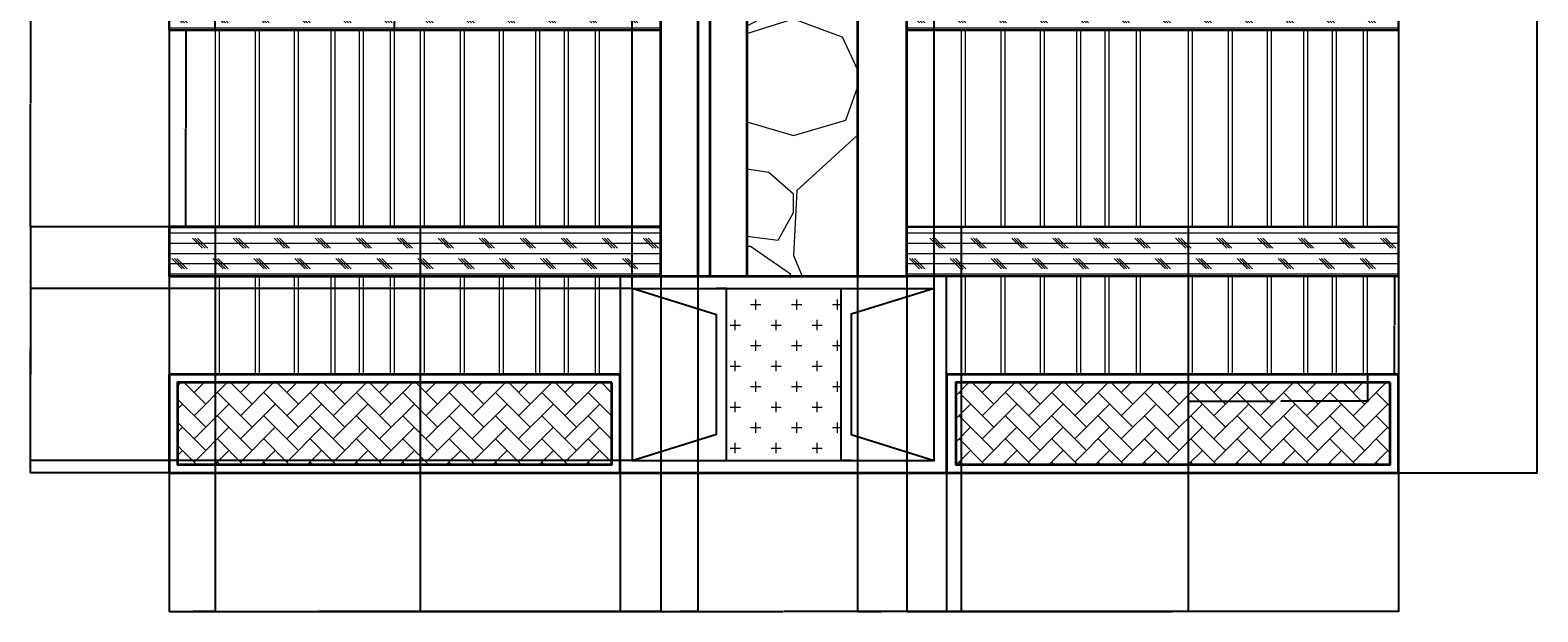
# Model space of a CAD drawing. Units: inches. Extents: x -38 to 698, y -57 to 1364.
# Tile 1 of 5: x -38 to 698, y -57 to 227. Entities that reach past the tile are written whole.
import ezdxf

# ---------------------------------------------------------------- set-up
doc = ezdxf.new("R2010")
doc.units = ezdxf.units.IN
doc.header["$MEASUREMENT"] = 0
for name, color, linetype, lineweight in [('A-ANNO-DIMS', 2, 'Continuous', 18), ('A-DOOR', 3, 'Continuous', 25), ('A-DOOR-PATT', 8, 'Continuous', 13), ('A-ELEV-PATT', 8, 'Continuous', 13), ('A-ELEV-SCRN', 7, 'Continuous', 20), ('A-FLOR', 7, 'Continuous', 30), ('A-WALL', 7, 'Continuous', 35), ('A-WALL-PATT', 8, 'Continuous', 13)]:
    doc.layers.add(name, color=color, linetype=linetype, lineweight=lineweight)
doc.styles.get("Standard").update_dxf_attribs({"font": 'arial.ttf'})
doc.dimstyles.get("Standard").update_dxf_attribs({"dimtxt": 0.18, "dimasz": 0.18, "dimexe": 0.18, "dimexo": 0.0625, "dimgap": 0.09, "dimtad": 0, "dimtih": 1, "dimtoh": 1, "dimdec": 4, "dimzin": 0, "dimdsep": 46, "dimtxsty": 'Standard', "dimcen": 0.09, "dimadec": 0, "dimazin": 0, "dimtfac": 1, "dimtdec": 4, "dimtofl": 0, "dimtmove": 0, "dimatfit": 3, "dimfxl": 1, "dimtolj": 1, "dimtzin": 0, "dimarcsym": 0})

# ---------------------------------------------------------------- blocks, each defined once
blk = doc.blocks.new('PODIUM-SCREEN-48')
for points in [[(0, 0), (2.11, 0), (2.11, 48), (0, 48)], [(19.49, 0), (21.6, 0), (21.6, 48), (19.49, 48)], [(38.57, 0), (40.67, 0), (40.67, 48), (38.57, 48)], [(56.37, 0), (58.48, 0), (58.48, 48), (56.37, 48)], [(70.28, 0), (72.39, 0), (72.39, 48), (70.28, 48)], [(85.45, 0), (87.56, 0), (87.56, 48), (85.45, 48)]]:
    blk.add_lwpolyline(points, close=True)
blk = doc.blocks.new('PODIUM-SCREEN-96')
for points in [[(0, 0), (2.11, 0), (2.11, 96), (0, 96)], [(19.49, 0), (21.6, 0), (21.6, 96), (19.49, 96)], [(38.57, 0), (40.67, 0), (40.67, 96), (38.57, 96)], [(56.37, 0), (58.48, 0), (58.48, 96), (56.37, 96)], [(70.28, 0), (72.39, 0), (72.39, 96), (70.28, 96)], [(85.45, 0), (87.56, 0), (87.56, 96), (85.45, 96)]]:
    blk.add_lwpolyline(points, close=True)
blk = doc.blocks.new('*D18')
at = {"layer": 'A-ANNO-DIMS', "color": 0, "lineweight": -2, "transparency": 16777216}
for p, q in [((527.04, 59.15), (527.04, 45.9)), ((614.61, 59.15), (614.61, 45.9)), ((527.22, 46.08), (569.42, 46.08)), ((614.43, 46.08), (572.23, 46.08))]:
    blk.add_line(p, q, dxfattribs=at)
at = {"layer": 'A-ANNO-DIMS', "color": 0, "transparency": 16777216}
for points in [[(527.22, 46.11), (527.22, 46.05), (527.04, 46.08)], [(614.43, 46.11), (614.43, 46.05), (614.61, 46.08)]]:
    blk.add_solid(points, dxfattribs=at)
at = {"layer": 'Defpoints', "color": 0, "transparency": 16777216}
for p in [(527.04, 59.21), (614.61, 59.21), (614.61, 46.08)]:
    blk.add_point(p, dxfattribs=at)
at = {"layer": 'A-ANNO-DIMS', "color": 0, "transparency": 16777216, "insert": (570.82, 46.08), "char_height": 0.18, "attachment_point": 5}
blk.add_mtext('\\A1;LOW SCREEN 88 TYP.', dxfattribs=at)
blk = doc.blocks.new('*D19')
at = {"layer": 'A-ANNO-DIMS', "color": 0, "lineweight": -2, "transparency": 16777216}
for p, q in [((614.67, 107.21), (627.92, 107.21)), ((627.74, 107.03), (627.74, 83.4)), ((627.74, 59.39), (627.74, 83.03)), ((614.67, 59.21), (627.92, 59.21))]:
    blk.add_line(p, q, dxfattribs=at)
at = {"layer": 'A-ANNO-DIMS', "color": 0, "transparency": 16777216}
for points in [[(627.71, 107.03), (627.77, 107.03), (627.74, 107.21)], [(627.71, 59.39), (627.77, 59.39), (627.74, 59.21)]]:
    blk.add_solid(points, dxfattribs=at)
at = {"layer": 'Defpoints', "color": 0, "transparency": 16777216}
for p in [(614.61, 107.21), (627.74, 107.21), (614.61, 59.21)]:
    blk.add_point(p, dxfattribs=at)
at = {"layer": 'A-ANNO-DIMS', "color": 0, "transparency": 16777216, "insert": (627.74, 83.21), "char_height": 0.18, "attachment_point": 5}
blk.add_mtext('\\A1;48 TYP.', dxfattribs=at)
blk = doc.blocks.new('*D20')
at = {"layer": 'A-ANNO-DIMS', "color": 0, "lineweight": -2, "transparency": 16777216}
for p, q in [((52.08, 227.21), (37.56, 227.21)), ((37.74, 227.03), (37.74, 179.4)), ((37.74, 131.39), (37.74, 179.03)), ((52.08, 131.21), (37.56, 131.21))]:
    blk.add_line(p, q, dxfattribs=at)
at = {"layer": 'A-ANNO-DIMS', "color": 0, "transparency": 16777216}
for points in [[(37.71, 227.03), (37.77, 227.03), (37.74, 227.21)], [(37.71, 131.39), (37.77, 131.39), (37.74, 131.21)]]:
    blk.add_solid(points, dxfattribs=at)
at = {"layer": 'Defpoints', "color": 0, "transparency": 16777216}
for p in [(37.74, 227.21), (52.14, 227.21), (52.14, 131.21)]:
    blk.add_point(p, dxfattribs=at)
at = {"layer": 'A-ANNO-DIMS', "color": 0, "transparency": 16777216, "insert": (37.74, 179.21), "char_height": 0.18, "attachment_point": 5}
blk.add_mtext('\\A1;HIGH SCREEN 96 TYP.', dxfattribs=at)
blk = doc.blocks.new('*D21')
at = {"layer": 'A-ANNO-DIMS', "color": 0, "lineweight": -2, "transparency": 16777216}
for p, q in [((52.14, 227.28), (52.14, 241.79)), ((52.32, 241.61), (95.39, 241.61)), ((139.52, 241.61), (96.45, 241.61)), ((139.7, 227.28), (139.7, 241.79))]:
    blk.add_line(p, q, dxfattribs=at)
at = {"layer": 'A-ANNO-DIMS', "color": 0, "transparency": 16777216}
for points in [[(52.32, 241.64), (52.32, 241.58), (52.14, 241.61)], [(139.52, 241.64), (139.52, 241.58), (139.7, 241.61)]]:
    blk.add_solid(points, dxfattribs=at)
at = {"layer": 'Defpoints', "color": 0, "transparency": 16777216}
for p in [(139.7, 241.61), (52.14, 227.21), (139.7, 227.21)]:
    blk.add_point(p, dxfattribs=at)
at = {"layer": 'A-ANNO-DIMS', "color": 0, "transparency": 16777216, "insert": (95.92, 241.61), "char_height": 0.18, "attachment_point": 5}
blk.add_mtext('\\A1;88 TYP.', dxfattribs=at)
blk = doc.blocks.new('*D22')
at = {"layer": 'A-ANNO-DIMS', "color": 0, "lineweight": -2, "transparency": 16777216}
for p, q in [((29.69, 500.15), (29.69, -56.67)), ((629.69, 500.15), (629.69, -56.67)), ((29.87, -56.49), (329.4, -56.49)), ((629.51, -56.49), (329.97, -56.49))]:
    blk.add_line(p, q, dxfattribs=at)
at = {"layer": 'A-ANNO-DIMS', "color": 0, "transparency": 16777216}
for points in [[(29.87, -56.46), (29.87, -56.52), (29.69, -56.49)], [(629.51, -56.46), (629.51, -56.52), (629.69, -56.49)]]:
    blk.add_solid(points, dxfattribs=at)
at = {"layer": 'Defpoints', "color": 0, "transparency": 16777216}
for p in [(29.69, 500.21), (629.69, 500.21), (629.69, -56.49)]:
    blk.add_point(p, dxfattribs=at)
at = {"layer": 'A-ANNO-DIMS', "color": 0, "transparency": 16777216, "insert": (329.69, -56.49), "char_height": 0.18, "attachment_point": 5}
blk.add_mtext('\\A1;600', dxfattribs=at)
blk = doc.blocks.new('*D23')
at = {"layer": 'A-ANNO-DIMS', "color": 0, "lineweight": -2, "transparency": 16777216}
for p, q in [((595.72, 1295.04), (697.57, 1295.04)), ((697.39, 1294.86), (697.39, 653.31)), ((697.39, 11.39), (697.39, 652.94)), ((629.75, 11.21), (697.57, 11.21))]:
    blk.add_line(p, q, dxfattribs=at)
at = {"layer": 'A-ANNO-DIMS', "color": 0, "transparency": 16777216}
for points in [[(697.36, 1294.86), (697.42, 1294.86), (697.39, 1295.04)], [(697.36, 11.39), (697.42, 11.39), (697.39, 11.21)]]:
    blk.add_solid(points, dxfattribs=at)
at = {"layer": 'Defpoints', "color": 0, "transparency": 16777216}
for p in [(595.66, 1295.04), (697.39, 1295.04), (629.69, 11.21)]:
    blk.add_point(p, dxfattribs=at)
at = {"layer": 'A-ANNO-DIMS', "color": 0, "transparency": 16777216, "insert": (697.39, 653.13), "char_height": 0.18, "attachment_point": 5}
blk.add_mtext('\\A1;1283.8', dxfattribs=at)
blk = doc.blocks.new('*D24')
at = {"layer": 'A-ANNO-DIMS', "color": 0, "lineweight": -2, "transparency": 16777216}
for p, q in [((29.69, 1100.15), (29.69, -56.67)), ((269.69, 1100.15), (269.69, -56.67)), ((29.87, -56.49), (149.4, -56.49)), ((269.51, -56.49), (149.98, -56.49))]:
    blk.add_line(p, q, dxfattribs=at)
at = {"layer": 'A-ANNO-DIMS', "color": 0, "transparency": 16777216}
for points in [[(29.87, -56.46), (29.87, -56.52), (29.69, -56.49)], [(269.51, -56.46), (269.51, -56.52), (269.69, -56.49)]]:
    blk.add_solid(points, dxfattribs=at)
at = {"layer": 'Defpoints', "color": 0, "transparency": 16777216}
for p in [(29.69, 1100.21), (269.69, 1100.21), (269.69, -56.49)]:
    blk.add_point(p, dxfattribs=at)
at = {"layer": 'A-ANNO-DIMS', "color": 0, "transparency": 16777216, "insert": (149.69, -56.49), "char_height": 0.18, "attachment_point": 5}
blk.add_mtext('\\A1;240', dxfattribs=at)
blk = doc.blocks.new('*D25')
at = {"layer": 'A-ANNO-DIMS', "color": 0, "lineweight": -2, "transparency": 16777216}
for p, q in [((269.69, 1100.15), (269.69, -56.67)), ((389.69, 1100.15), (389.69, -56.67)), ((269.87, -56.49), (329.41, -56.49)), ((389.51, -56.49), (329.97, -56.49))]:
    blk.add_line(p, q, dxfattribs=at)
at = {"layer": 'A-ANNO-DIMS', "color": 0, "transparency": 16777216}
for points in [[(269.87, -56.46), (269.87, -56.52), (269.69, -56.49)], [(389.51, -56.46), (389.51, -56.52), (389.69, -56.49)]]:
    blk.add_solid(points, dxfattribs=at)
at = {"layer": 'Defpoints', "color": 0, "transparency": 16777216}
for p in [(269.69, 1100.21), (389.69, 1100.21), (389.69, -56.49)]:
    blk.add_point(p, dxfattribs=at)
at = {"layer": 'A-ANNO-DIMS', "color": 0, "transparency": 16777216, "insert": (329.69, -56.49), "char_height": 0.18, "attachment_point": 5}
blk.add_mtext('\\A1;120', dxfattribs=at)
blk = doc.blocks.new('*D26')
at = {"layer": 'A-ANNO-DIMS', "color": 0, "lineweight": -2, "transparency": 16777216}
for p, q in [((389.69, 1100.15), (389.69, -56.67)), ((629.69, 1100.15), (629.69, -56.67)), ((389.87, -56.49), (509.4, -56.49)), ((629.51, -56.49), (509.98, -56.49))]:
    blk.add_line(p, q, dxfattribs=at)
at = {"layer": 'A-ANNO-DIMS', "color": 0, "transparency": 16777216}
for points in [[(389.87, -56.46), (389.87, -56.52), (389.69, -56.49)], [(629.51, -56.46), (629.51, -56.52), (629.69, -56.49)]]:
    blk.add_solid(points, dxfattribs=at)
at = {"layer": 'Defpoints', "color": 0, "transparency": 16777216}
for p in [(389.69, 1100.21), (629.69, 1100.21), (629.69, -56.49)]:
    blk.add_point(p, dxfattribs=at)
at = {"layer": 'A-ANNO-DIMS', "color": 0, "transparency": 16777216, "insert": (509.69, -56.49), "char_height": 0.18, "attachment_point": 5}
blk.add_mtext('\\A1;240', dxfattribs=at)
blk = doc.blocks.new('*D29')
at = {"layer": 'A-ANNO-DIMS', "color": 0, "lineweight": -2, "transparency": 16777216}
for p, q in [((29.62, 131.21), (-38.19, 131.21)), ((-38.01, 131.03), (-38.01, 71.4)), ((-38.01, 11.39), (-38.01, 71.03)), ((29.62, 11.21), (-38.19, 11.21))]:
    blk.add_line(p, q, dxfattribs=at)
at = {"layer": 'A-ANNO-DIMS', "color": 0, "transparency": 16777216}
for points in [[(-38.04, 131.03), (-37.98, 131.03), (-38.01, 131.21)], [(-38.04, 11.39), (-37.98, 11.39), (-38.01, 11.21)]]:
    blk.add_solid(points, dxfattribs=at)
at = {"layer": 'Defpoints', "color": 0, "transparency": 16777216}
for p in [(-38.01, 131.21), (29.69, 131.21), (29.69, 11.21)]:
    blk.add_point(p, dxfattribs=at)
at = {"layer": 'A-ANNO-DIMS', "color": 0, "transparency": 16777216, "insert": (-38.01, 71.21), "char_height": 0.18, "attachment_point": 5}
blk.add_mtext('\\A1;120', dxfattribs=at)
blk = doc.blocks.new('*D30')
at = {"layer": 'A-ANNO-DIMS', "color": 0, "lineweight": -2, "transparency": 16777216}
for p, q in [((29.62, 251.21), (-38.19, 251.21)), ((-38.01, 251.03), (-38.01, 191.4)), ((-38.01, 131.39), (-38.01, 191.03)), ((29.62, 131.21), (-38.19, 131.21))]:
    blk.add_line(p, q, dxfattribs=at)
at = {"layer": 'A-ANNO-DIMS', "color": 0, "transparency": 16777216}
for points in [[(-38.04, 251.03), (-37.98, 251.03), (-38.01, 251.21)], [(-38.04, 131.39), (-37.98, 131.39), (-38.01, 131.21)]]:
    blk.add_solid(points, dxfattribs=at)
at = {"layer": 'Defpoints', "color": 0, "transparency": 16777216}
for p in [(-38.01, 251.21), (29.69, 251.21), (29.69, 131.21)]:
    blk.add_point(p, dxfattribs=at)
at = {"layer": 'A-ANNO-DIMS', "color": 0, "transparency": 16777216, "insert": (-38.01, 191.21), "char_height": 0.18, "attachment_point": 5}
blk.add_mtext('\\A1;120', dxfattribs=at)
blk = doc.blocks.new('*D40')
at = {"layer": 'A-ANNO-DIMS', "color": 0, "lineweight": -2, "transparency": 16777216}
for p, q in [((249.72, 11.15), (249.72, -56.67)), ((409.03, 11.15), (409.03, -56.67)), ((249.9, -56.49), (328.99, -56.49)), ((408.85, -56.49), (329.76, -56.49))]:
    blk.add_line(p, q, dxfattribs=at)
at = {"layer": 'A-ANNO-DIMS', "color": 0, "transparency": 16777216}
for points in [[(249.9, -56.46), (249.9, -56.52), (249.72, -56.49)], [(408.85, -56.46), (408.85, -56.52), (409.03, -56.49)]]:
    blk.add_solid(points, dxfattribs=at)
at = {"layer": 'Defpoints', "color": 0, "transparency": 16777216}
for p in [(249.72, 11.21), (409.03, 11.21), (409.03, -56.49)]:
    blk.add_point(p, dxfattribs=at)
at = {"layer": 'A-ANNO-DIMS', "color": 0, "transparency": 16777216, "insert": (329.37, -56.49), "char_height": 0.18, "attachment_point": 5}
blk.add_mtext('\\A1;159.3', dxfattribs=at)
blk = doc.blocks.new('*D41')
at = {"layer": 'A-ANNO-DIMS', "color": 0, "lineweight": -2, "transparency": 16777216}
for p, q in [((29.69, 11.15), (29.69, -56.67)), ((249.72, 11.15), (249.72, -56.67)), ((29.87, -56.49), (139.24, -56.49)), ((249.54, -56.49), (140.17, -56.49))]:
    blk.add_line(p, q, dxfattribs=at)
at = {"layer": 'A-ANNO-DIMS', "color": 0, "transparency": 16777216}
for points in [[(29.87, -56.46), (29.87, -56.52), (29.69, -56.49)], [(249.54, -56.46), (249.54, -56.52), (249.72, -56.49)]]:
    blk.add_solid(points, dxfattribs=at)
at = {"layer": 'Defpoints', "color": 0, "transparency": 16777216}
for p in [(29.69, 11.21), (249.72, 11.21), (249.72, -56.49)]:
    blk.add_point(p, dxfattribs=at)
at = {"layer": 'A-ANNO-DIMS', "color": 0, "transparency": 16777216, "insert": (139.7, -56.49), "char_height": 0.18, "attachment_point": 5}
blk.add_mtext('\\A1;220.03', dxfattribs=at)
blk = doc.blocks.new('*D42')
at = {"layer": 'A-ANNO-DIMS', "color": 0, "lineweight": -2, "transparency": 16777216}
for p, q in [((409.03, 11.15), (409.03, -56.67)), ((629.69, 11.15), (629.69, -56.67)), ((409.21, -56.49), (518.89, -56.49)), ((629.51, -56.49), (519.82, -56.49))]:
    blk.add_line(p, q, dxfattribs=at)
at = {"layer": 'A-ANNO-DIMS', "color": 0, "transparency": 16777216}
for points in [[(409.21, -56.46), (409.21, -56.52), (409.03, -56.49)], [(629.51, -56.46), (629.51, -56.52), (629.69, -56.49)]]:
    blk.add_solid(points, dxfattribs=at)
at = {"layer": 'Defpoints', "color": 0, "transparency": 16777216}
for p in [(409.03, 11.21), (629.69, 11.21), (629.69, -56.49)]:
    blk.add_point(p, dxfattribs=at)
at = {"layer": 'A-ANNO-DIMS', "color": 0, "transparency": 16777216, "insert": (519.36, -56.49), "char_height": 0.18, "attachment_point": 5}
blk.add_mtext('\\A1;220.66', dxfattribs=at)
blk = doc.blocks.new('*D47')
at = {"layer": 'A-ANNO-DIMS', "color": 0, "lineweight": -2, "transparency": 16777216}
for p, q in [((255.66, 101.21), (-38.19, 101.21)), ((-38.01, 101.03), (-38.01, 59.4)), ((-38.01, 17.39), (-38.01, 59.03)), ((255.66, 17.21), (-38.19, 17.21))]:
    blk.add_line(p, q, dxfattribs=at)
at = {"layer": 'A-ANNO-DIMS', "color": 0, "transparency": 16777216}
for points in [[(-38.04, 101.03), (-37.98, 101.03), (-38.01, 101.21)], [(-38.04, 17.39), (-37.98, 17.39), (-38.01, 17.21)]]:
    blk.add_solid(points, dxfattribs=at)
at = {"layer": 'Defpoints', "color": 0, "transparency": 16777216}
for p in [(-38.01, 101.21), (255.72, 101.21), (255.72, 17.21)]:
    blk.add_point(p, dxfattribs=at)
at = {"layer": 'A-ANNO-DIMS', "color": 0, "transparency": 16777216, "insert": (-38.01, 59.21), "char_height": 0.18, "attachment_point": 5}
blk.add_mtext('\\A1;84', dxfattribs=at)
blk = doc.blocks.new('*D48')
at = {"layer": 'A-ANNO-DIMS', "color": 0, "lineweight": -2, "transparency": 16777216}
for p, q in [((255.72, 101.28), (255.72, 1362.92)), ((255.9, 1362.74), (328.99, 1362.74)), ((402.85, 1362.74), (329.76, 1362.74)), ((403.03, 101.28), (403.03, 1362.92))]:
    blk.add_line(p, q, dxfattribs=at)
at = {"layer": 'A-ANNO-DIMS', "color": 0, "transparency": 16777216}
for points in [[(255.9, 1362.77), (255.9, 1362.71), (255.72, 1362.74)], [(402.85, 1362.77), (402.85, 1362.71), (403.03, 1362.74)]]:
    blk.add_solid(points, dxfattribs=at)
at = {"layer": 'Defpoints', "color": 0, "transparency": 16777216}
for p in [(403.03, 1362.74), (255.72, 101.21), (403.03, 101.21)]:
    blk.add_point(p, dxfattribs=at)
at = {"layer": 'A-ANNO-DIMS', "color": 0, "transparency": 16777216, "insert": (329.37, 1362.74), "char_height": 0.18, "attachment_point": 5}
blk.add_mtext('\\A1;147.3', dxfattribs=at)
blk = doc.blocks.new('*D51')
at = {"layer": 'A-ANNO-DIMS', "color": 0, "lineweight": -2, "transparency": 16777216}
for p, q in [((365.69, 1294.97), (365.69, -56.67)), ((389.69, 1258.97), (389.69, -56.67)), ((365.87, -56.49), (377.47, -56.49)), ((389.51, -56.49), (377.91, -56.49))]:
    blk.add_line(p, q, dxfattribs=at)
at = {"layer": 'A-ANNO-DIMS', "color": 0, "transparency": 16777216}
for points in [[(365.87, -56.46), (365.87, -56.52), (365.69, -56.49)], [(389.51, -56.46), (389.51, -56.52), (389.69, -56.49)]]:
    blk.add_solid(points, dxfattribs=at)
at = {"layer": 'Defpoints', "color": 0, "transparency": 16777216}
for p in [(365.69, 1295.04), (389.69, 1259.04), (389.69, -56.49)]:
    blk.add_point(p, dxfattribs=at)
at = {"layer": 'A-ANNO-DIMS', "color": 0, "transparency": 16777216, "insert": (377.69, -56.49), "char_height": 0.18, "attachment_point": 5}
blk.add_mtext('\\A1;24', dxfattribs=at)
blk = doc.blocks.new('*D52')
at = {"layer": 'A-ANNO-DIMS', "color": 0, "lineweight": -2, "transparency": 16777216}
for p, q in [((287.69, 1294.97), (287.69, -56.67)), ((269.69, 1282.97), (269.69, -56.67)), ((269.87, -56.49), (278.47, -56.49)), ((287.51, -56.49), (278.9, -56.49))]:
    blk.add_line(p, q, dxfattribs=at)
at = {"layer": 'A-ANNO-DIMS', "color": 0, "transparency": 16777216}
for points in [[(269.87, -56.46), (269.87, -56.52), (269.69, -56.49)], [(287.51, -56.46), (287.51, -56.52), (287.69, -56.49)]]:
    blk.add_solid(points, dxfattribs=at)
at = {"layer": 'Defpoints', "color": 0, "transparency": 16777216}
for p in [(287.69, 1295.04), (269.69, 1283.04), (287.69, -56.49)]:
    blk.add_point(p, dxfattribs=at)
at = {"layer": 'A-ANNO-DIMS', "color": 0, "transparency": 16777216, "insert": (278.69, -56.49), "char_height": 0.18, "attachment_point": 5}
blk.add_mtext('\\A1;18', dxfattribs=at)
blk = doc.blocks.new('*D55')
at = {"layer": 'A-ANNO-DIMS', "color": 0, "lineweight": -2, "transparency": 16777216}
for p, q in [((29.69, 131.15), (29.69, -56.67)), ((52.14, 131.15), (52.14, -56.67)), ((29.87, -56.49), (40.45, -56.49)), ((51.96, -56.49), (41.38, -56.49))]:
    blk.add_line(p, q, dxfattribs=at)
at = {"layer": 'A-ANNO-DIMS', "color": 0, "transparency": 16777216}
for points in [[(29.87, -56.46), (29.87, -56.52), (29.69, -56.49)], [(51.96, -56.46), (51.96, -56.52), (52.14, -56.49)]]:
    blk.add_solid(points, dxfattribs=at)
at = {"layer": 'Defpoints', "color": 0, "transparency": 16777216}
for p in [(29.69, 131.21), (52.14, 131.21), (52.14, -56.49)]:
    blk.add_point(p, dxfattribs=at)
at = {"layer": 'A-ANNO-DIMS', "color": 0, "transparency": 16777216, "insert": (40.91, -56.49), "char_height": 0.18, "attachment_point": 5}
blk.add_mtext('\\A1;22.455', dxfattribs=at)
blk = doc.blocks.new('*D56')
at = {"layer": 'A-ANNO-DIMS', "color": 0, "lineweight": -2, "transparency": 16777216}
for p, q in [((52.14, 131.15), (52.14, -56.67)), ((152.18, 131.15), (152.18, -56.67)), ((52.32, -56.49), (101.7, -56.49)), ((152, -56.49), (102.61, -56.49))]:
    blk.add_line(p, q, dxfattribs=at)
at = {"layer": 'A-ANNO-DIMS', "color": 0, "transparency": 16777216}
for points in [[(52.32, -56.46), (52.32, -56.52), (52.14, -56.49)], [(152, -56.46), (152, -56.52), (152.18, -56.49)]]:
    blk.add_solid(points, dxfattribs=at)
at = {"layer": 'Defpoints', "color": 0, "transparency": 16777216}
for p in [(52.14, 131.21), (152.18, 131.21), (152.18, -56.49)]:
    blk.add_point(p, dxfattribs=at)
at = {"layer": 'A-ANNO-DIMS', "color": 0, "transparency": 16777216, "insert": (102.16, -56.49), "char_height": 0.18, "attachment_point": 5}
blk.add_mtext('\\A1;100.03', dxfattribs=at)
blk = doc.blocks.new('*D57')
at = {"layer": 'A-ANNO-DIMS', "color": 0, "lineweight": -2, "transparency": 16777216}
for p, q in [((389.69, 131.15), (389.69, -56.67)), ((416.19, 131.15), (416.19, -56.67)), ((389.87, -56.49), (402.61, -56.49)), ((416.01, -56.49), (403.26, -56.49))]:
    blk.add_line(p, q, dxfattribs=at)
at = {"layer": 'A-ANNO-DIMS', "color": 0, "transparency": 16777216}
for points in [[(389.87, -56.46), (389.87, -56.52), (389.69, -56.49)], [(416.01, -56.46), (416.01, -56.52), (416.19, -56.49)]]:
    blk.add_solid(points, dxfattribs=at)
at = {"layer": 'Defpoints', "color": 0, "transparency": 16777216}
for p in [(389.69, 131.21), (416.19, 131.21), (416.19, -56.49)]:
    blk.add_point(p, dxfattribs=at)
at = {"layer": 'A-ANNO-DIMS', "color": 0, "transparency": 16777216, "insert": (402.94, -56.49), "char_height": 0.18, "attachment_point": 5}
blk.add_mtext('\\A1;26.5', dxfattribs=at)
blk = doc.blocks.new('*D58')
at = {"layer": 'A-ANNO-DIMS', "color": 0, "lineweight": -2, "transparency": 16777216}
for p, q in [((416.19, 131.15), (416.19, -56.67)), ((527.04, 131.15), (527.04, -56.67)), ((416.37, -56.49), (471.16, -56.49)), ((526.86, -56.49), (472.07, -56.49))]:
    blk.add_line(p, q, dxfattribs=at)
at = {"layer": 'A-ANNO-DIMS', "color": 0, "transparency": 16777216}
for points in [[(416.37, -56.46), (416.37, -56.52), (416.19, -56.49)], [(526.86, -56.46), (526.86, -56.52), (527.04, -56.49)]]:
    blk.add_solid(points, dxfattribs=at)
at = {"layer": 'Defpoints', "color": 0, "transparency": 16777216}
for p in [(416.19, 131.21), (527.04, 131.21), (527.04, -56.49)]:
    blk.add_point(p, dxfattribs=at)
at = {"layer": 'A-ANNO-DIMS', "color": 0, "transparency": 16777216, "insert": (471.61, -56.49), "char_height": 0.18, "attachment_point": 5}
blk.add_mtext('\\A1;110.86', dxfattribs=at)

msp = doc.modelspace()

# ---------------------------------------------------------------- hatches: boundary and pattern name
at = {"layer": 'A-DOOR-PATT', "transparency": 33554562}
h = msp.add_hatch(dxfattribs=at)
h.set_pattern_fill('CROSS', color=256, scale=40)
h.set_pattern_definition([(0, (-116.553, -96.733), (10, 10), [5, -15]), (90, (-114.053, -99.233), (-10, 10), [5, -15])])
h.paths.add_polyline_path([(357.7018, 101.2149), (301.6691, 101.2149), (301.6691, 17.2149), (357.7018, 17.2149)])
at = {"layer": 'A-ELEV-PATT', "transparency": 33554562}
h = msp.add_hatch(dxfattribs=at)
h.set_pattern_fill('CORK', color=256, scale=40)
h.set_pattern_definition([(0, (-116.5534, -96.733), (0, 5), []), (135, (-114.053, -99.233), (-10, -10), [7.07107, -7.07107]), (135, (-112.803, -99.233), (-10, -10), [7.07107, -7.07107]), (135, (-111.553, -99.233), (-10, -10), [7.07107, -7.07107])])
h.paths.add_polyline_path([(269.6854, 131.2149), (29.6854, 131.2149), (29.6854, 107.2149), (269.6854, 107.2149)])
h.paths.add_polyline_path([(269.6854, 251.2149), (29.6854, 251.2149), (29.6854, 227.2149), (269.6854, 227.2149)])
h.paths.add_polyline_path([(629.6854, 251.2149), (389.6854, 251.2149), (389.6854, 227.2149), (629.6854, 227.2149)])
h.paths.add_polyline_path([(629.6854, 131.2149), (389.6854, 131.2149), (389.6854, 107.2149), (409.029, 107.2149), (629.6854, 107.2149)])
at = {"layer": 'A-WALL-PATT', "transparency": 33554625}
h = msp.add_hatch(dxfattribs=at)
h.set_pattern_fill('GRAVEL', color=256, scale=150)
h.set_pattern_definition([(228.0128, (-8.553, 53.267), (-1200, -1350), [20.1804, -1997.863]), (184.96974, (-22.0534, 38.267), (1800, 150), [34.63, -3428.3887]), (132.51045, (-56.553, 35.267), (1500, -1650), [24.418, -2417.405]), (267.2737, (-115.0534, -2.233), (150, 3000), [31.5357, -3122.0337]), (292.83365, (-116.5534, -33.733), (-750, 1800), [30.923, -3061.406]), (357.2737, (-104.5534, -62.233), (-3000, 150), [31.5357, -3122.0337]), (37.69424, (-73.0534, -63.733), (-1950, -1500), [41.7043, -4128.7273]), (72.25533, (-40.0534, -38.233), (1050, 3300), [39.373, -3897.9482]), (121.42957, (-28.0534, -0.733), (-1200, 1950), [31.6425, -3132.611]), (175.2364, (-44.553, 26.267), (1650, -150), [36.125, -1770.1144]), (222.39744, (-80.5534, 29.267), (-1800, -1650), [46.7172, -4625.0063]), (138.8141, (33.447, -3.733), (-1050, 900), [15.945, -1578.577]), (171.4692, (21.447, 6.767), (1950, -300), [30.3356, -3003.2267]), (225, (-8.55, 11.27), (-2e-14, -150), [21.213, -190.919]), (203.1986, (-19.053, 29.267), (750, 300), [11.424, -1130.942]), (291.8014, (-29.553, 24.767), (-150, 450), [16.155, -791.619]), (30.9638, (-23.553, 9.767), (450, 300), [26.239, -848.403]), (161.565, (-1.053, 23.267), (300, -150), [18.974, -455.368]), (16.38954, (-116.553, 24.767), (1500, 450), [26.58, -2631.427]), (70.3462, (-91.053, 32.267), (-600, -1650), [22.299, -2207.611]), (293.1986, (-1.053, 53.267), (-300, 750), [22.847, -1119.519]), (343.6105, (7.947, 32.267), (-1500, 450), [26.58, -2631.427]), (339.444, (-116.553, -68.233), (-750, 300), [25.632, -1255.9686]), (294.7751, (-92.553, -77.233), (-750, 1650), [21.477, -2126.1965]), (66.8014, (0.447, -96.733), (300, 750), [22.847, -1119.519]), (17.354, (9.447, -75.733), (-1950, -600), [25.1446, -2489.3135]), (69.444, (-73.053, -96.733), (-300, -750), [12.816, -1268.7846]), (101.31, (-8.553, -96.733), (-150, 600), [7.649, -757.204]), (165.9638, (-10.053, -89.233), (450, -150), [30.923, -587.543]), (186.009, (-40.053, -81.733), (1500, 150), [28.6575, -2837.0885]), (303.69, (-23.553, -3.733), (-150, 300), [21.633, -519.2]), (353.1572, (-11.5534, -21.733), (2550, -300), [37.769, -3739.1344]), (60.9454, (25.947, -26.233), (-600, -1050), [15.443, -1528.901]), (90, (33.45, -12.73), (-150, 150), [9, -141]), (120.2564, (-43.053, -77.233), (600, -1050), [20.8386, -2063.028]), (48.0128, (-53.553, -59.233), (1200, 1350), [40.361, -1977.683]), (0, (-26.55, -29.23), (150, 150), [39, -111]), (325.30485, (12.447, -29.233), (1500, -1050), [23.717, -2347.991]), (254.0546, (31.947, -42.733), (-150, -600), [21.84, -1070.176]), (207.646, (25.9466, -63.733), (-2850, -1500), [35.5598, -3520.421]), (175.4261, (-5.5534, -80.233), (-1950, 150), [37.62, -3724.361])])
h.paths.add_polyline_path([(311.6854, 107.2149), (365.6854, 107.2149), (365.6854, 851.2149), (365.6854, 971.2149), (365.6854, 1091.2149), (365.6854, 1140.6923), (311.6854, 1140.6923), (311.6854, 971.2149), (311.6854, 851.2149)])
h = msp.add_hatch(dxfattribs=at)
h.set_pattern_fill('AR-HBONE', color=256, scale=2)
h.set_pattern_definition([(45, (-116.553, -96.733), (0, 11.31371), [24, -8]), (135, (-110.8965, -91.076), (9e-16, 11.31371), [24, -8])])
h.paths.add_polyline_path([(245.7202, 55.2149), (33.6854, 55.2149), (33.6854, 15.2149), (245.7202, 15.2149)])
h.paths.add_polyline_path([(625.6854, 55.2149), (413.6507, 55.2149), (413.6507, 15.2149), (625.6854, 15.2149)])

# ---------------------------------------------------------------- linework, layer by layer
at = {"layer": 'A-DOOR'}
msp.add_line((255.7202, 17.2149), (403.029, 17.2149), dxfattribs=at)
msp.add_lwpolyline([(249.7202, 11.2149), (409.029, 11.2149), (409.029, 107.2149), (249.7202, 107.2149)], close=True, dxfattribs=at)
for points in [[(255.7202, 101.2149), (255.7202, 17.2149), (296.8108, 30.0679), (296.8108, 88.3619), (255.7202, 101.2149), (403.029, 101.2149), (362.5601, 88.5563), (362.5601, 29.8735), (403.029, 17.2149), (403.029, 101.2149)], [(296.8108, 17.2149), (301.6691, 17.2149), (301.6691, 101.2149), (296.8108, 101.2149)], [(362.5601, 17.2149), (357.7018, 17.2149), (357.7018, 101.2149), (362.5601, 101.2149)]]:
    msp.add_lwpolyline(points, dxfattribs=at)
at = {"layer": 'A-FLOR'}
for points in [[(29.6854, 296.3406), (29.6854, 251.2149), (29.6854, 227.2149), (269.6854, 227.2149)], [(629.0638, 227.2149), (389.6854, 227.2149), (629.6854, 227.2149), (629.6854, 251.2149), (389.6854, 251.2149), (629.6854, 251.2149)], [(389.6854, 107.2149), (629.6854, 107.2149), (629.6854, 131.2149), (389.6854, 131.2149), (629.6854, 131.2149)]]:
    msp.add_lwpolyline(points, dxfattribs=at)
at = {"layer": 'A-WALL'}
msp.add_line((29.6854, 11.2149), (629.6854, 11.2149), dxfattribs=at)
for points in [[(29.6854, 131.2149), (269.6854, 131.2149), (29.6854, 131.2149), (29.6854, 107.2149), (389.6854, 107.2149), (389.6854, 851.2149), (389.6854, 971.2149), (389.6854, 1091.2149), (389.6854, 1259.0353), (595.6569, 1259.0353), (595.6569, 1295.0353), (365.6854, 1295.0353), (365.6854, 1211.2149), (365.6854, 1091.2149), (365.6854, 971.2149), (365.6854, 851.2149), (365.6854, 107.2149)], [(269.6854, 107.2149), (269.6854, 851.2149), (269.6854, 971.2149), (269.6854, 1283.0353), (141.3895, 1283.0353), (141.3895, 1295.0353), (287.6854, 1295.0353), (287.6854, 971.2149), (287.6854, 851.2149), (287.6854, 107.2149)], [(293.6854, 107.2149), (293.6854, 851.2149), (293.6854, 971.2149), (293.6854, 1295.0353), (311.6854, 1295.0353), (311.6854, 1211.2149), (311.6854, 971.2149), (311.6854, 851.2149), (311.6854, 107.2149)], [(29.6854, 59.2149), (29.6854, 11.2149)], [(629.6854, 11.2149), (629.6854, 59.2149)]]:
    msp.add_lwpolyline(points, dxfattribs=at)
for points in [[(249.7202, 59.2149), (29.6854, 59.2149), (29.6854, 11.2149), (249.7202, 11.2149)], [(629.6854, 59.2149), (409.029, 59.2149), (409.029, 11.2149), (629.6854, 11.2149)], [(245.7202, 55.2149), (33.6854, 55.2149), (33.6854, 15.2149), (245.7202, 15.2149)], [(625.6854, 55.2149), (413.6507, 55.2149), (413.6507, 15.2149), (625.6854, 15.2149)]]:
    msp.add_lwpolyline(points, close=True, dxfattribs=at)

# ---------------------------------------------------------------- block references
at = {"layer": 'A-ELEV-SCRN'}
for name, p in [('PODIUM-SCREEN-96', (52.141, 131.215)), ('PODIUM-SCREEN-96', (152.1758, 131.215)), ('PODIUM-SCREEN-96', (416.1852, 131.215)), ('PODIUM-SCREEN-96', (527.0432, 131.215)), ('PODIUM-SCREEN-48', (52.141, 59.215)), ('PODIUM-SCREEN-48', (152.1758, 59.215)), ('PODIUM-SCREEN-48', (416.1852, 59.215)), ('PODIUM-SCREEN-48', (527.0432, 59.215))]:
    msp.add_blockref(name, p, dxfattribs=at)

# ---------------------------------------------------------------- dimensions: what is measured, and where the dimension line sits
at = {"layer": 'A-ANNO-DIMS'}
for base, p1, p2, override, picture, middle in [((403.029, 1362.7353), (255.7202, 101.2149), (403.029, 101.2149), {"dimdec": 1, "dimlfac": 1, "dimrnd": 0, "dimzin": 0, "dimdsep": 46, "dimlunit": 2}, '*D48', (329.3746, 1362.7353)), ((287.6854, -56.4851), (269.6854, 1283.0353), (287.6854, 1295.0353), {"dimdec": 0, "dimlfac": 1, "dimrnd": 0, "dimzin": 0, "dimdsep": 46, "dimlunit": 2}, '*D52', (278.6854, -56.4851)), ((389.6854, -56.4851), (365.6854, 1295.0353), (389.6854, 1259.0353), {"dimdec": 0, "dimlfac": 1, "dimrnd": 0, "dimzin": 0, "dimdsep": 46, "dimlunit": 2}, '*D51', (377.6854, -56.4851)), ((269.6854, -56.4851), (29.6854, 1100.2149), (269.6854, 1100.2149), {"dimdec": 0, "dimlfac": 1, "dimrnd": 0, "dimzin": 0, "dimdsep": 46, "dimlunit": 2}, '*D24', (149.6854, -56.4851)), ((389.6854, -56.4851), (269.6854, 1100.2149), (389.6854, 1100.2149), {"dimdec": 0, "dimlfac": 1, "dimrnd": 0, "dimzin": 0, "dimdsep": 46, "dimlunit": 2}, '*D25', (329.6854, -56.4851)), ((629.6854, -56.4851), (389.6854, 1100.2149), (629.6854, 1100.2149), {"dimdec": 0, "dimlfac": 1, "dimrnd": 0, "dimzin": 0, "dimdsep": 46, "dimlunit": 2}, '*D26', (509.6854, -56.4851)), ((629.6854, -56.4851), (29.6854, 500.2149), (629.6854, 500.2149), {"dimdec": 0, "dimlfac": 1, "dimrnd": 0, "dimzin": 0, "dimdsep": 46, "dimlunit": 2}, '*D22', (329.6854, -56.4851)), ((52.1408, -56.4851), (29.6854, 131.2149), (52.1408, 131.2149), {"dimdec": 3, "dimlfac": 1, "dimrnd": 0, "dimzin": 0, "dimdsep": 46, "dimlunit": 2}, '*D55', (40.9131, -56.4851)), ((152.1756, -56.4851), (52.1408, 131.2149), (152.1756, 131.2149), {"dimdec": 2, "dimlfac": 1, "dimrnd": 0, "dimzin": 0, "dimdsep": 46, "dimlunit": 2}, '*D56', (102.1582, -56.4851)), ((416.1851, -56.4851), (389.6854, 131.2149), (416.1851, 131.2149), {"dimdec": 1, "dimlfac": 1, "dimrnd": 0, "dimzin": 0, "dimdsep": 46, "dimlunit": 2}, '*D57', (402.9353, -56.4851)), ((527.043, -56.4851), (416.1851, 131.2149), (527.043, 131.2149), {"dimdec": 2, "dimlfac": 1, "dimrnd": 0, "dimzin": 0, "dimdsep": 46, "dimlunit": 2}, '*D58', (471.614, -56.4851)), ((249.7202, -56.4851), (29.6854, 11.2149), (249.7202, 11.2149), {"dimdec": 2, "dimlfac": 1, "dimrnd": 0, "dimzin": 0, "dimdsep": 46, "dimlunit": 2}, '*D41', (139.7028, -56.4851)), ((409.029, -56.4851), (249.7202, 11.2149), (409.029, 11.2149), {"dimdec": 1, "dimlfac": 1, "dimrnd": 0, "dimzin": 0, "dimdsep": 46, "dimlunit": 2}, '*D40', (329.3746, -56.4851)), ((629.6854, -56.4851), (409.029, 11.2149), (629.6854, 11.2149), {"dimdec": 2, "dimlfac": 1, "dimrnd": 0, "dimzin": 0, "dimdsep": 46, "dimlunit": 2}, '*D42', (519.3572, -56.4851))]:
    dim = msp.add_linear_dim(base=base, p1=p1, p2=p2, dimstyle='Standard', override=override, dxfattribs=at)
    dim.commit()
    dim.dimension.update_dxf_attribs({"geometry": picture, "text_midpoint": middle})
for base, p1, p2, override, picture, middle in [((697.3854, 1295.0353), (629.6854, 11.2149), (595.6569, 1295.0353), {"dimdec": 1, "dimlfac": 1, "dimrnd": 0, "dimzin": 0, "dimdsep": 46, "dimlunit": 2}, '*D23', (697.3854, 653.1251)), ((-38.0146, 251.2149), (29.6854, 131.2149), (29.6854, 251.2149), {"dimdec": 0, "dimlfac": 1, "dimrnd": 0, "dimzin": 0, "dimdsep": 46, "dimlunit": 2}, '*D30', (-38.0146, 191.2149)), ((-38.0146, 131.2149), (29.6854, 11.2149), (29.6854, 131.2149), {"dimdec": 0, "dimlfac": 1, "dimrnd": 0, "dimzin": 0, "dimdsep": 46, "dimlunit": 2}, '*D29', (-38.0146, 71.2149)), ((-38.0146, 101.2149), (255.7202, 17.2149), (255.7202, 101.2149), {"dimdec": 0, "dimlfac": 1, "dimrnd": 0, "dimzin": 0, "dimdsep": 46, "dimlunit": 2}, '*D47', (-38.0146, 59.2149))]:
    dim = msp.add_linear_dim(base=base, p1=p1, p2=p2, angle=90, dimstyle='Standard', override=override, dxfattribs=at)
    dim.commit()
    dim.dimension.update_dxf_attribs({"geometry": picture, "text_midpoint": middle})
for base, p1, p2, text, picture, middle in [((139.7028, 241.6149), (52.1408, 227.2149), (139.7028, 227.2149), '<> TYP.', '*D21', (95.9218, 241.6149)), ((614.605, 46.0806), (527.043, 59.2149), (614.605, 59.2149), 'LOW SCREEN <> TYP.', '*D18', (570.824, 46.0806))]:
    dim = msp.add_linear_dim(base=base, p1=p1, p2=p2, text=text, dimstyle='Standard', override={"dimdec": 0, "dimlfac": 1, "dimrnd": 0, "dimzin": 0, "dimdsep": 46, "dimlunit": 2}, dxfattribs=at)
    dim.commit()
    dim.dimension.update_dxf_attribs({"geometry": picture, "text_midpoint": middle})
for base, p1, p2, text, picture, middle in [((37.7408, 227.2149), (52.1408, 131.2149), (52.1408, 227.2149), 'HIGH SCREEN <> TYP.', '*D20', (37.7408, 179.2149)), ((627.7393, 107.2149), (614.605, 59.2149), (614.605, 107.2149), '<> TYP.', '*D19', (627.7393, 83.2149))]:
    dim = msp.add_linear_dim(base=base, p1=p1, p2=p2, angle=90, text=text, dimstyle='Standard', override={"dimdec": 0, "dimlfac": 1, "dimrnd": 0, "dimzin": 0, "dimdsep": 46, "dimlunit": 2}, dxfattribs=at)
    dim.commit()
    dim.dimension.update_dxf_attribs({"geometry": picture, "text_midpoint": middle})

doc.saveas('drawing.dxf')
